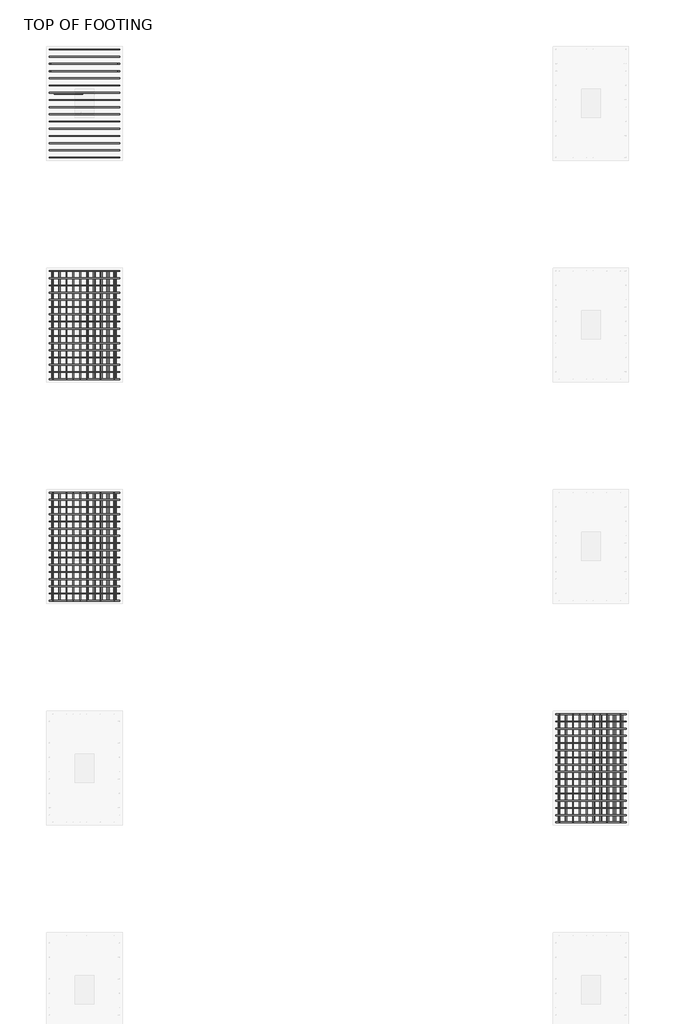
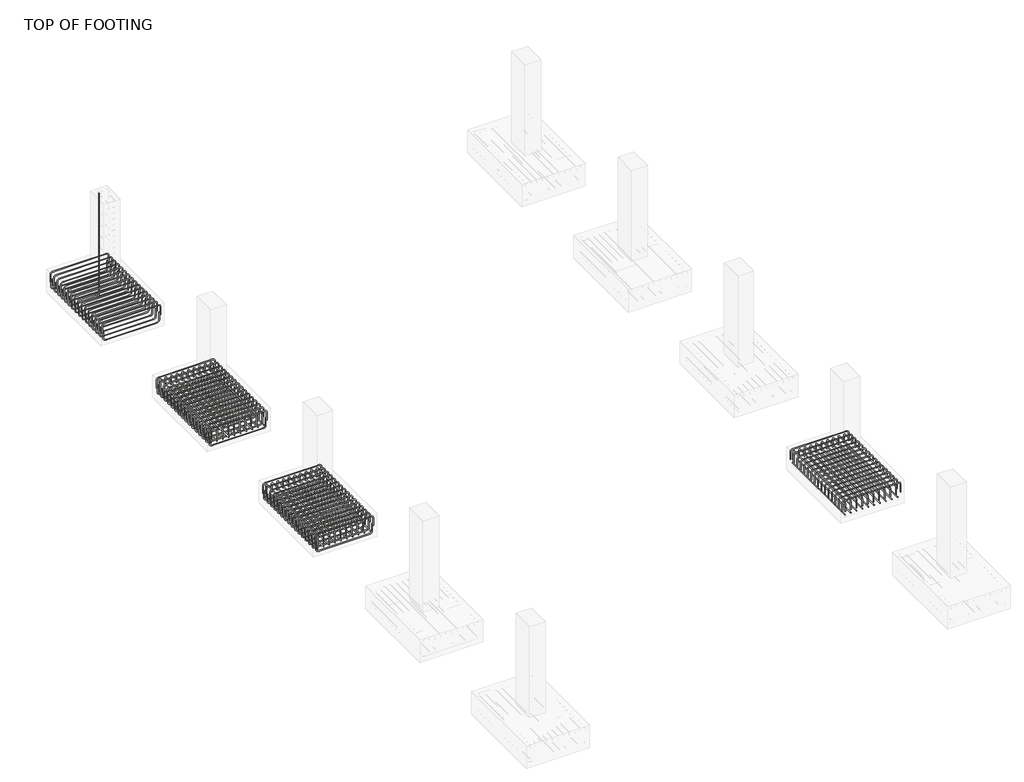
# One storey, part 3 of 8: 14 reinforcing bars.
"""IFC4 building model written with IfcOpenShell, lengths in millimetres."""

from ifc_helpers import new_model, si_unit, point, frame, origin, place, context, project, spatial, polyline, circle_curve, trimmed, segment, composite_curve, source, transform, mapped, element, save
from ifc_brep_helpers import swept_disk

model = new_model("IFC4")

# Units and contexts
model_context = context("Model", 3, world=origin())
ifc_project = project(units=[si_unit("LENGTHUNIT", "METRE", prefix="MILLI")], contexts=[model_context])

# Site, building, storey
site = spatial("IfcSite", under=ifc_project)
building = spatial("IfcBuilding", under=site)
storey = spatial("IfcBuildingStorey", under=building, Name="TOP OF FOOTING", Elevation=-1828.8)

# Reinforcing bars
placement = place(None, origin())
reinforcing_bar_shape = source(origin(), model_context, "Body", "SolidModel", [
    swept_disk(composite_curve([segment(polyline([(-11301.5220197, 16626.3508557, -2021.4413313), (-11301.5220197, 16626.3508557, -2168.7413313)]), True, "CONTINUOUS"), segment(trimmed(circle_curve(frame((-11347.8720197, 16626.3508557, -2168.7413313), z_axis=(0.0, 1.0, 0.0), x_axis=(46.350000000000364, 0.0, 0.0)), 46.35), [point((-11301.5220197, 16626.3508557, -2168.7413313))], [point((-11347.8720197, 16626.3508557, -2215.0913313))], True, "CARTESIAN"), True, "CONTINUOUS"), segment(polyline([(-11347.8720197, 16626.3508557, -2215.0913313), (-12320.167031, 16626.3508557, -2215.0913313)]), True, "CONTINUOUS"), segment(trimmed(circle_curve(frame((-12320.167031, 16626.3508557, -2168.7413313), z_axis=(0.0, 1.0, 0.0), x_axis=(0.0, 0.0, -46.34999999999991)), 46.35), [point((-12320.167031, 16626.3508557, -2215.0913313))], [point((-12366.517031, 16626.3508557, -2168.7413313))], True, "CARTESIAN"), True, "CONTINUOUS"), segment(polyline([(-12366.517031, 16626.3508557, -2168.7413313), (-12366.517031, 16626.3508557, -2021.4413313)]), True, "CONTINUOUS")], self_intersect=False), 6.35),
])
element("IfcReinforcingBar", 1, at=placement, inside=storey, context=model_context, shape_type="MappedRepresentation", body=[
    mapped(reinforcing_bar_shape, transform((0.0, 0.0, 0.0), x_axis=(1.0, 0.0, 0.0), y_axis=(0.0, 1.0, 0.0), z_axis=(0.0, 0.0, 1.0))),
    mapped(reinforcing_bar_shape, transform((0.0, -113.82, 0.0), x_axis=(1.0, 0.0, 0.0), y_axis=(0.0, 1.0, 0.0), z_axis=(0.0, 0.0, 1.0))),
    mapped(reinforcing_bar_shape, transform((0.0, -227.64, 0.0), x_axis=(1.0, 0.0, 0.0), y_axis=(0.0, 1.0, 0.0), z_axis=(0.0, 0.0, 1.0))),
    mapped(reinforcing_bar_shape, transform((0.0, -341.46, 0.0), x_axis=(1.0, 0.0, 0.0), y_axis=(0.0, 1.0, 0.0), z_axis=(0.0, 0.0, 1.0))),
    mapped(reinforcing_bar_shape, transform((0.0, -455.28, 0.0), x_axis=(1.0, 0.0, 0.0), y_axis=(0.0, 1.0, 0.0), z_axis=(0.0, 0.0, 1.0))),
    mapped(reinforcing_bar_shape, transform((0.0, -569.1, 0.0), x_axis=(1.0, 0.0, 0.0), y_axis=(0.0, 1.0, 0.0), z_axis=(0.0, 0.0, 1.0))),
    mapped(reinforcing_bar_shape, transform((0.0, -682.92, 0.0), x_axis=(1.0, 0.0, 0.0), y_axis=(0.0, 1.0, 0.0), z_axis=(0.0, 0.0, 1.0))),
    mapped(reinforcing_bar_shape, transform((0.0, -796.74, 0.0), x_axis=(1.0, 0.0, 0.0), y_axis=(0.0, 1.0, 0.0), z_axis=(0.0, 0.0, 1.0))),
    mapped(reinforcing_bar_shape, transform((0.0, -910.56, 0.0), x_axis=(1.0, 0.0, 0.0), y_axis=(0.0, 1.0, 0.0), z_axis=(0.0, 0.0, 1.0))),
    mapped(reinforcing_bar_shape, transform((0.0, -1024.38, 0.0), x_axis=(1.0, 0.0, 0.0), y_axis=(0.0, 1.0, 0.0), z_axis=(0.0, 0.0, 1.0))),
    mapped(reinforcing_bar_shape, transform((0.0, -1138.2, 0.0), x_axis=(1.0, 0.0, 0.0), y_axis=(0.0, 1.0, 0.0), z_axis=(0.0, 0.0, 1.0))),
    mapped(reinforcing_bar_shape, transform((0.0, -1252.02, 0.0), x_axis=(1.0, 0.0, 0.0), y_axis=(0.0, 1.0, 0.0), z_axis=(0.0, 0.0, 1.0))),
    mapped(reinforcing_bar_shape, transform((0.0, -1365.84, 0.0), x_axis=(1.0, 0.0, 0.0), y_axis=(0.0, 1.0, 0.0), z_axis=(0.0, 0.0, 1.0))),
    mapped(reinforcing_bar_shape, transform((0.0, -1479.66, 0.0), x_axis=(1.0, 0.0, 0.0), y_axis=(0.0, 1.0, 0.0), z_axis=(0.0, 0.0, 1.0))),
    mapped(reinforcing_bar_shape, transform((0.0, -1593.48, 0.0), x_axis=(1.0, 0.0, 0.0), y_axis=(0.0, 1.0, 0.0), z_axis=(0.0, 0.0, 1.0))),
    mapped(reinforcing_bar_shape, transform((0.0, -1707.3, 0.0), x_axis=(1.0, 0.0, 0.0), y_axis=(0.0, 1.0, 0.0), z_axis=(0.0, 0.0, 1.0))),
])
reinforcing_bar_2_shape = source(origin(), model_context, "Body", "SolidModel", [
    swept_disk(composite_curve([segment(polyline([(-12384.3374017, 16626.3508557, -2068.8), (-12384.3374017, 16626.3508557, -1921.5)]), True, "CONTINUOUS"), segment(trimmed(circle_curve(frame((-12337.9874017, 16626.3508557, -1921.5), z_axis=(0.0, 1.0, 0.0), x_axis=(-46.350000000000364, 0.0, 0.0)), 46.35), [point((-12384.3374017, 16626.3508557, -1921.5))], [point((-12337.9874017, 16626.3508557, -1875.15))], True, "CARTESIAN"), True, "CONTINUOUS"), segment(polyline([(-12337.9874017, 16626.3508557, -1875.15), (-11323.3874017, 16626.3508557, -1875.15)]), True, "CONTINUOUS"), segment(trimmed(circle_curve(frame((-11323.3874017, 16626.3508557, -1921.5), z_axis=(0.0, 1.0, 0.0), x_axis=(0.0, 0.0, 46.34999999999991)), 46.35), [point((-11323.3874017, 16626.3508557, -1875.15))], [point((-11277.0374017, 16626.3508557, -1921.5))], True, "CARTESIAN"), True, "CONTINUOUS"), segment(polyline([(-11277.0374017, 16626.3508557, -1921.5), (-11277.0374017, 16626.3508557, -2068.8)]), True, "CONTINUOUS")], self_intersect=False), 6.35),
])
element("IfcReinforcingBar", 2, at=placement, inside=storey, context=model_context, shape_type="MappedRepresentation", body=[
    mapped(reinforcing_bar_2_shape, transform((0.0, 0.0, 0.0), x_axis=(1.0, 0.0, 0.0), y_axis=(0.0, 1.0, 0.0), z_axis=(0.0, 0.0, 1.0))),
    mapped(reinforcing_bar_2_shape, transform((0.0, -113.82, 0.0), x_axis=(1.0, 0.0, 0.0), y_axis=(0.0, 1.0, 0.0), z_axis=(0.0, 0.0, 1.0))),
    mapped(reinforcing_bar_2_shape, transform((0.0, -227.64, 0.0), x_axis=(1.0, 0.0, 0.0), y_axis=(0.0, 1.0, 0.0), z_axis=(0.0, 0.0, 1.0))),
    mapped(reinforcing_bar_2_shape, transform((0.0, -341.46, 0.0), x_axis=(1.0, 0.0, 0.0), y_axis=(0.0, 1.0, 0.0), z_axis=(0.0, 0.0, 1.0))),
    mapped(reinforcing_bar_2_shape, transform((0.0, -455.28, 0.0), x_axis=(1.0, 0.0, 0.0), y_axis=(0.0, 1.0, 0.0), z_axis=(0.0, 0.0, 1.0))),
    mapped(reinforcing_bar_2_shape, transform((0.0, -569.1, 0.0), x_axis=(1.0, 0.0, 0.0), y_axis=(0.0, 1.0, 0.0), z_axis=(0.0, 0.0, 1.0))),
    mapped(reinforcing_bar_2_shape, transform((0.0, -682.92, 0.0), x_axis=(1.0, 0.0, 0.0), y_axis=(0.0, 1.0, 0.0), z_axis=(0.0, 0.0, 1.0))),
    mapped(reinforcing_bar_2_shape, transform((0.0, -796.74, 0.0), x_axis=(1.0, 0.0, 0.0), y_axis=(0.0, 1.0, 0.0), z_axis=(0.0, 0.0, 1.0))),
    mapped(reinforcing_bar_2_shape, transform((0.0, -910.56, 0.0), x_axis=(1.0, 0.0, 0.0), y_axis=(0.0, 1.0, 0.0), z_axis=(0.0, 0.0, 1.0))),
    mapped(reinforcing_bar_2_shape, transform((0.0, -1024.38, 0.0), x_axis=(1.0, 0.0, 0.0), y_axis=(0.0, 1.0, 0.0), z_axis=(0.0, 0.0, 1.0))),
    mapped(reinforcing_bar_2_shape, transform((0.0, -1138.2, 0.0), x_axis=(1.0, 0.0, 0.0), y_axis=(0.0, 1.0, 0.0), z_axis=(0.0, 0.0, 1.0))),
    mapped(reinforcing_bar_2_shape, transform((0.0, -1252.02, 0.0), x_axis=(1.0, 0.0, 0.0), y_axis=(0.0, 1.0, 0.0), z_axis=(0.0, 0.0, 1.0))),
    mapped(reinforcing_bar_2_shape, transform((0.0, -1365.84, 0.0), x_axis=(1.0, 0.0, 0.0), y_axis=(0.0, 1.0, 0.0), z_axis=(0.0, 0.0, 1.0))),
    mapped(reinforcing_bar_2_shape, transform((0.0, -1479.66, 0.0), x_axis=(1.0, 0.0, 0.0), y_axis=(0.0, 1.0, 0.0), z_axis=(0.0, 0.0, 1.0))),
    mapped(reinforcing_bar_2_shape, transform((0.0, -1593.48, 0.0), x_axis=(1.0, 0.0, 0.0), y_axis=(0.0, 1.0, 0.0), z_axis=(0.0, 0.0, 1.0))),
    mapped(reinforcing_bar_2_shape, transform((0.0, -1707.3, 0.0), x_axis=(1.0, 0.0, 0.0), y_axis=(0.0, 1.0, 0.0), z_axis=(0.0, 0.0, 1.0))),
])
element("IfcReinforcingBar", 3, at=placement, inside=storey, context=model_context, shape_type="SolidModel", body=[
    swept_disk(composite_curve([segment(polyline([(-11865.9367429, 15924.2508557, -40.0), (-11865.9367429, 15924.2508557, -2055.5685723)]), True, "CONTINUOUS"), segment(trimmed(circle_curve(frame((-11912.2867429, 15924.2508557, -2055.5685723), z_axis=(0.0, 1.0, 0.0), x_axis=(46.350000000000364, 0.0, 0.0)), 46.35), [point((-11865.9367429, 15924.2508557, -2055.5685723))], [point((-11912.2867429, 15924.2508557, -2101.9185723))], True, "CARTESIAN"), True, "CONTINUOUS"), segment(polyline([(-11912.2867429, 15924.2508557, -2101.9185723), (-12306.1579683, 15924.2508557, -2101.9185723)]), True, "CONTINUOUS")], self_intersect=False), 6.35),
])
reinforcing_bar_3_shape = source(origin(), model_context, "Body", "SolidModel", [
    swept_disk(composite_curve([segment(polyline([(-11301.5220197, 13126.3508557, -2021.4413313), (-11301.5220197, 13126.3508557, -2168.7413313)]), True, "CONTINUOUS"), segment(trimmed(circle_curve(frame((-11347.8720197, 13126.3508557, -2168.7413313), z_axis=(0.0, 1.0, 0.0), x_axis=(46.350000000000364, 0.0, 0.0)), 46.35), [point((-11301.5220197, 13126.3508557, -2168.7413313))], [point((-11347.8720197, 13126.3508557, -2215.0913313))], True, "CARTESIAN"), True, "CONTINUOUS"), segment(polyline([(-11347.8720197, 13126.3508557, -2215.0913313), (-12320.167031, 13126.3508557, -2215.0913313)]), True, "CONTINUOUS"), segment(trimmed(circle_curve(frame((-12320.167031, 13126.3508557, -2168.7413313), z_axis=(0.0, 1.0, 0.0), x_axis=(0.0, 0.0, -46.34999999999991)), 46.35), [point((-12320.167031, 13126.3508557, -2215.0913313))], [point((-12366.517031, 13126.3508557, -2168.7413313))], True, "CARTESIAN"), True, "CONTINUOUS"), segment(polyline([(-12366.517031, 13126.3508557, -2168.7413313), (-12366.517031, 13126.3508557, -2021.4413313)]), True, "CONTINUOUS")], self_intersect=False), 6.35),
])
element("IfcReinforcingBar", 4, at=placement, inside=storey, context=model_context, shape_type="MappedRepresentation", body=[
    mapped(reinforcing_bar_3_shape, transform((0.0, 0.0, 0.0), x_axis=(1.0, 0.0, 0.0), y_axis=(0.0, 1.0, 0.0), z_axis=(0.0, 0.0, 1.0))),
    mapped(reinforcing_bar_3_shape, transform((0.0, -113.82, 0.0), x_axis=(1.0, 0.0, 0.0), y_axis=(0.0, 1.0, 0.0), z_axis=(0.0, 0.0, 1.0))),
    mapped(reinforcing_bar_3_shape, transform((0.0, -227.64, 0.0), x_axis=(1.0, 0.0, 0.0), y_axis=(0.0, 1.0, 0.0), z_axis=(0.0, 0.0, 1.0))),
    mapped(reinforcing_bar_3_shape, transform((0.0, -341.46, 0.0), x_axis=(1.0, 0.0, 0.0), y_axis=(0.0, 1.0, 0.0), z_axis=(0.0, 0.0, 1.0))),
    mapped(reinforcing_bar_3_shape, transform((0.0, -455.28, 0.0), x_axis=(1.0, 0.0, 0.0), y_axis=(0.0, 1.0, 0.0), z_axis=(0.0, 0.0, 1.0))),
    mapped(reinforcing_bar_3_shape, transform((0.0, -569.1, 0.0), x_axis=(1.0, 0.0, 0.0), y_axis=(0.0, 1.0, 0.0), z_axis=(0.0, 0.0, 1.0))),
    mapped(reinforcing_bar_3_shape, transform((0.0, -682.92, 0.0), x_axis=(1.0, 0.0, 0.0), y_axis=(0.0, 1.0, 0.0), z_axis=(0.0, 0.0, 1.0))),
    mapped(reinforcing_bar_3_shape, transform((0.0, -796.74, 0.0), x_axis=(1.0, 0.0, 0.0), y_axis=(0.0, 1.0, 0.0), z_axis=(0.0, 0.0, 1.0))),
    mapped(reinforcing_bar_3_shape, transform((0.0, -910.56, 0.0), x_axis=(1.0, 0.0, 0.0), y_axis=(0.0, 1.0, 0.0), z_axis=(0.0, 0.0, 1.0))),
    mapped(reinforcing_bar_3_shape, transform((0.0, -1024.38, 0.0), x_axis=(1.0, 0.0, 0.0), y_axis=(0.0, 1.0, 0.0), z_axis=(0.0, 0.0, 1.0))),
    mapped(reinforcing_bar_3_shape, transform((0.0, -1138.2, 0.0), x_axis=(1.0, 0.0, 0.0), y_axis=(0.0, 1.0, 0.0), z_axis=(0.0, 0.0, 1.0))),
    mapped(reinforcing_bar_3_shape, transform((0.0, -1252.02, 0.0), x_axis=(1.0, 0.0, 0.0), y_axis=(0.0, 1.0, 0.0), z_axis=(0.0, 0.0, 1.0))),
    mapped(reinforcing_bar_3_shape, transform((0.0, -1365.84, 0.0), x_axis=(1.0, 0.0, 0.0), y_axis=(0.0, 1.0, 0.0), z_axis=(0.0, 0.0, 1.0))),
    mapped(reinforcing_bar_3_shape, transform((0.0, -1479.66, 0.0), x_axis=(1.0, 0.0, 0.0), y_axis=(0.0, 1.0, 0.0), z_axis=(0.0, 0.0, 1.0))),
    mapped(reinforcing_bar_3_shape, transform((0.0, -1593.48, 0.0), x_axis=(1.0, 0.0, 0.0), y_axis=(0.0, 1.0, 0.0), z_axis=(0.0, 0.0, 1.0))),
    mapped(reinforcing_bar_3_shape, transform((0.0, -1707.3, 0.0), x_axis=(1.0, 0.0, 0.0), y_axis=(0.0, 1.0, 0.0), z_axis=(0.0, 0.0, 1.0))),
])
reinforcing_bar_4_shape = source(origin(), model_context, "Body", "SolidModel", [
    swept_disk(composite_curve([segment(polyline([(-12384.3374017, 13126.3508557, -2068.8), (-12384.3374017, 13126.3508557, -1921.5)]), True, "CONTINUOUS"), segment(trimmed(circle_curve(frame((-12337.9874017, 13126.3508557, -1921.5), z_axis=(0.0, 1.0, 0.0), x_axis=(-46.350000000000364, 0.0, 0.0)), 46.35), [point((-12384.3374017, 13126.3508557, -1921.5))], [point((-12337.9874017, 13126.3508557, -1875.15))], True, "CARTESIAN"), True, "CONTINUOUS"), segment(polyline([(-12337.9874017, 13126.3508557, -1875.15), (-11323.3874017, 13126.3508557, -1875.15)]), True, "CONTINUOUS"), segment(trimmed(circle_curve(frame((-11323.3874017, 13126.3508557, -1921.5), z_axis=(0.0, 1.0, 0.0), x_axis=(0.0, 0.0, 46.34999999999991)), 46.35), [point((-11323.3874017, 13126.3508557, -1875.15))], [point((-11277.0374017, 13126.3508557, -1921.5))], True, "CARTESIAN"), True, "CONTINUOUS"), segment(polyline([(-11277.0374017, 13126.3508557, -1921.5), (-11277.0374017, 13126.3508557, -2068.8)]), True, "CONTINUOUS")], self_intersect=False), 6.35),
])
element("IfcReinforcingBar", 5, at=placement, inside=storey, context=model_context, shape_type="MappedRepresentation", body=[
    mapped(reinforcing_bar_4_shape, transform((0.0, 0.0, 0.0), x_axis=(1.0, 0.0, 0.0), y_axis=(0.0, 1.0, 0.0), z_axis=(0.0, 0.0, 1.0))),
    mapped(reinforcing_bar_4_shape, transform((0.0, -113.82, 0.0), x_axis=(1.0, 0.0, 0.0), y_axis=(0.0, 1.0, 0.0), z_axis=(0.0, 0.0, 1.0))),
    mapped(reinforcing_bar_4_shape, transform((0.0, -227.64, 0.0), x_axis=(1.0, 0.0, 0.0), y_axis=(0.0, 1.0, 0.0), z_axis=(0.0, 0.0, 1.0))),
    mapped(reinforcing_bar_4_shape, transform((0.0, -341.46, 0.0), x_axis=(1.0, 0.0, 0.0), y_axis=(0.0, 1.0, 0.0), z_axis=(0.0, 0.0, 1.0))),
    mapped(reinforcing_bar_4_shape, transform((0.0, -455.28, 0.0), x_axis=(1.0, 0.0, 0.0), y_axis=(0.0, 1.0, 0.0), z_axis=(0.0, 0.0, 1.0))),
    mapped(reinforcing_bar_4_shape, transform((0.0, -569.1, 0.0), x_axis=(1.0, 0.0, 0.0), y_axis=(0.0, 1.0, 0.0), z_axis=(0.0, 0.0, 1.0))),
    mapped(reinforcing_bar_4_shape, transform((0.0, -682.92, 0.0), x_axis=(1.0, 0.0, 0.0), y_axis=(0.0, 1.0, 0.0), z_axis=(0.0, 0.0, 1.0))),
    mapped(reinforcing_bar_4_shape, transform((0.0, -796.74, 0.0), x_axis=(1.0, 0.0, 0.0), y_axis=(0.0, 1.0, 0.0), z_axis=(0.0, 0.0, 1.0))),
    mapped(reinforcing_bar_4_shape, transform((0.0, -910.56, 0.0), x_axis=(1.0, 0.0, 0.0), y_axis=(0.0, 1.0, 0.0), z_axis=(0.0, 0.0, 1.0))),
    mapped(reinforcing_bar_4_shape, transform((0.0, -1024.38, 0.0), x_axis=(1.0, 0.0, 0.0), y_axis=(0.0, 1.0, 0.0), z_axis=(0.0, 0.0, 1.0))),
    mapped(reinforcing_bar_4_shape, transform((0.0, -1138.2, 0.0), x_axis=(1.0, 0.0, 0.0), y_axis=(0.0, 1.0, 0.0), z_axis=(0.0, 0.0, 1.0))),
    mapped(reinforcing_bar_4_shape, transform((0.0, -1252.02, 0.0), x_axis=(1.0, 0.0, 0.0), y_axis=(0.0, 1.0, 0.0), z_axis=(0.0, 0.0, 1.0))),
    mapped(reinforcing_bar_4_shape, transform((0.0, -1365.84, 0.0), x_axis=(1.0, 0.0, 0.0), y_axis=(0.0, 1.0, 0.0), z_axis=(0.0, 0.0, 1.0))),
    mapped(reinforcing_bar_4_shape, transform((0.0, -1479.66, 0.0), x_axis=(1.0, 0.0, 0.0), y_axis=(0.0, 1.0, 0.0), z_axis=(0.0, 0.0, 1.0))),
    mapped(reinforcing_bar_4_shape, transform((0.0, -1593.48, 0.0), x_axis=(1.0, 0.0, 0.0), y_axis=(0.0, 1.0, 0.0), z_axis=(0.0, 0.0, 1.0))),
    mapped(reinforcing_bar_4_shape, transform((0.0, -1707.3, 0.0), x_axis=(1.0, 0.0, 0.0), y_axis=(0.0, 1.0, 0.0), z_axis=(0.0, 0.0, 1.0))),
])
reinforcing_bar_5_shape = source(origin(), model_context, "Body", "SolidModel", [
    swept_disk(composite_curve([segment(polyline([(-12339.592709, 13132.7008557, -2155.1176129), (-12339.592709, 11412.7008557, -2155.1176129)]), True, "CONTINUOUS")], self_intersect=False), 6.35),
])
element("IfcReinforcingBar", 6, at=placement, inside=storey, context=model_context, shape_type="MappedRepresentation", body=[
    mapped(reinforcing_bar_5_shape, transform((0.0, 0.0, 0.0), x_axis=(1.0, 0.0, 0.0), y_axis=(0.0, 1.0, 0.0), z_axis=(0.0, 0.0, 1.0))),
    mapped(reinforcing_bar_5_shape, transform((111.602188, 0.0, 0.0), x_axis=(1.0, 0.0, 0.0), y_axis=(0.0, 1.0, 0.0), z_axis=(0.0, 0.0, 1.0))),
    mapped(reinforcing_bar_5_shape, transform((223.2043759, 0.0, 0.0), x_axis=(1.0, 0.0, 0.0), y_axis=(0.0, 1.0, 0.0), z_axis=(0.0, 0.0, 1.0))),
    mapped(reinforcing_bar_5_shape, transform((334.8065639, 0.0, 0.0), x_axis=(1.0, 0.0, 0.0), y_axis=(0.0, 1.0, 0.0), z_axis=(0.0, 0.0, 1.0))),
    mapped(reinforcing_bar_5_shape, transform((446.4087519, 0.0, 0.0), x_axis=(1.0, 0.0, 0.0), y_axis=(0.0, 1.0, 0.0), z_axis=(0.0, 0.0, 1.0))),
    mapped(reinforcing_bar_5_shape, transform((558.0109398, 0.0, 0.0), x_axis=(1.0, 0.0, 0.0), y_axis=(0.0, 1.0, 0.0), z_axis=(0.0, 0.0, 1.0))),
    mapped(reinforcing_bar_5_shape, transform((669.6131278, 0.0, 0.0), x_axis=(1.0, 0.0, 0.0), y_axis=(0.0, 1.0, 0.0), z_axis=(0.0, 0.0, 1.0))),
    mapped(reinforcing_bar_5_shape, transform((781.2153158, 0.0, 0.0), x_axis=(1.0, 0.0, 0.0), y_axis=(0.0, 1.0, 0.0), z_axis=(0.0, 0.0, 1.0))),
    mapped(reinforcing_bar_5_shape, transform((892.8175037, 0.0, 0.0), x_axis=(1.0, 0.0, 0.0), y_axis=(0.0, 1.0, 0.0), z_axis=(0.0, 0.0, 1.0))),
    mapped(reinforcing_bar_5_shape, transform((1004.4196917, 0.0, 0.0), x_axis=(1.0, 0.0, 0.0), y_axis=(0.0, 1.0, 0.0), z_axis=(0.0, 0.0, 1.0))),
])
reinforcing_bar_6_shape = source(origin(), model_context, "Body", "SolidModel", [
    swept_disk(composite_curve([segment(polyline([(-11364.2651981, 13126.3508557, -2094.6521303), (-11364.2651981, 13126.3508557, -1947.3521303)]), True, "CONTINUOUS"), segment(trimmed(circle_curve(frame((-11364.2651981, 13080.0008557, -1947.3521303), z_axis=(1.0, 0.0, 0.0), x_axis=(0.0, 46.350000000000364, 0.0)), 46.35), [point((-11364.2651981, 13126.3508557, -1947.3521303))], [point((-11364.2651981, 13080.0008557, -1901.0021303))], True, "CARTESIAN"), True, "CONTINUOUS"), segment(polyline([(-11364.2651981, 13080.0008557, -1901.0021303), (-11364.2651981, 11465.4008557, -1901.0021303)]), True, "CONTINUOUS"), segment(trimmed(circle_curve(frame((-11364.2651981, 11465.4008557, -1947.3521303), z_axis=(1.0, 0.0, 0.0), x_axis=(0.0, 0.0, 46.34999999999991)), 46.35), [point((-11364.2651981, 11465.4008557, -1901.0021303))], [point((-11364.2651981, 11419.0508557, -1947.3521303))], True, "CARTESIAN"), True, "CONTINUOUS"), segment(polyline([(-11364.2651981, 11419.0508557, -1947.3521303), (-11364.2651981, 11419.0508557, -2094.6521303)]), True, "CONTINUOUS")], self_intersect=False), 6.35),
])
element("IfcReinforcingBar", 7, at=placement, inside=storey, context=model_context, shape_type="MappedRepresentation", body=[
    mapped(reinforcing_bar_6_shape, transform((0.0, 0.0, 0.0), x_axis=(1.0, 0.0, 0.0), y_axis=(0.0, 1.0, 0.0), z_axis=(0.0, 0.0, 1.0))),
    mapped(reinforcing_bar_6_shape, transform((-107.1680233, 0.0, 0.0), x_axis=(1.0, 0.0, 0.0), y_axis=(0.0, 1.0, 0.0), z_axis=(0.0, 0.0, 1.0))),
    mapped(reinforcing_bar_6_shape, transform((-214.3360466, 0.0, 0.0), x_axis=(1.0, 0.0, 0.0), y_axis=(0.0, 1.0, 0.0), z_axis=(0.0, 0.0, 1.0))),
    mapped(reinforcing_bar_6_shape, transform((-321.5040699, 0.0, 0.0), x_axis=(1.0, 0.0, 0.0), y_axis=(0.0, 1.0, 0.0), z_axis=(0.0, 0.0, 1.0))),
    mapped(reinforcing_bar_6_shape, transform((-428.6720932, 0.0, 0.0), x_axis=(1.0, 0.0, 0.0), y_axis=(0.0, 1.0, 0.0), z_axis=(0.0, 0.0, 1.0))),
    mapped(reinforcing_bar_6_shape, transform((-535.8401165, 0.0, 0.0), x_axis=(1.0, 0.0, 0.0), y_axis=(0.0, 1.0, 0.0), z_axis=(0.0, 0.0, 1.0))),
    mapped(reinforcing_bar_6_shape, transform((-643.0081398, 0.0, 0.0), x_axis=(1.0, 0.0, 0.0), y_axis=(0.0, 1.0, 0.0), z_axis=(0.0, 0.0, 1.0))),
    mapped(reinforcing_bar_6_shape, transform((-750.176163, 0.0, 0.0), x_axis=(1.0, 0.0, 0.0), y_axis=(0.0, 1.0, 0.0), z_axis=(0.0, 0.0, 1.0))),
    mapped(reinforcing_bar_6_shape, transform((-857.3441863, 0.0, 0.0), x_axis=(1.0, 0.0, 0.0), y_axis=(0.0, 1.0, 0.0), z_axis=(0.0, 0.0, 1.0))),
    mapped(reinforcing_bar_6_shape, transform((-964.5122096, 0.0, 0.0), x_axis=(1.0, 0.0, 0.0), y_axis=(0.0, 1.0, 0.0), z_axis=(0.0, 0.0, 1.0))),
])
reinforcing_bar_7_shape = source(origin(), model_context, "Body", "SolidModel", [
    swept_disk(composite_curve([segment(polyline([(-11301.5220197, 9626.3508557, -2021.4413313), (-11301.5220197, 9626.3508557, -2168.7413313)]), True, "CONTINUOUS"), segment(trimmed(circle_curve(frame((-11347.8720197, 9626.3508557, -2168.7413313), z_axis=(0.0, 1.0, 0.0), x_axis=(46.350000000000364, 0.0, 0.0)), 46.35), [point((-11301.5220197, 9626.3508557, -2168.7413313))], [point((-11347.8720197, 9626.3508557, -2215.0913313))], True, "CARTESIAN"), True, "CONTINUOUS"), segment(polyline([(-11347.8720197, 9626.3508557, -2215.0913313), (-12320.167031, 9626.3508557, -2215.0913313)]), True, "CONTINUOUS"), segment(trimmed(circle_curve(frame((-12320.167031, 9626.3508557, -2168.7413313), z_axis=(0.0, 1.0, 0.0), x_axis=(0.0, 0.0, -46.34999999999991)), 46.35), [point((-12320.167031, 9626.3508557, -2215.0913313))], [point((-12366.517031, 9626.3508557, -2168.7413313))], True, "CARTESIAN"), True, "CONTINUOUS"), segment(polyline([(-12366.517031, 9626.3508557, -2168.7413313), (-12366.517031, 9626.3508557, -2021.4413313)]), True, "CONTINUOUS")], self_intersect=False), 6.35),
])
element("IfcReinforcingBar", 8, at=placement, inside=storey, context=model_context, shape_type="MappedRepresentation", body=[
    mapped(reinforcing_bar_7_shape, transform((0.0, 0.0, 0.0), x_axis=(1.0, 0.0, 0.0), y_axis=(0.0, 1.0, 0.0), z_axis=(0.0, 0.0, 1.0))),
    mapped(reinforcing_bar_7_shape, transform((0.0, -113.82, 0.0), x_axis=(1.0, 0.0, 0.0), y_axis=(0.0, 1.0, 0.0), z_axis=(0.0, 0.0, 1.0))),
    mapped(reinforcing_bar_7_shape, transform((0.0, -227.64, 0.0), x_axis=(1.0, 0.0, 0.0), y_axis=(0.0, 1.0, 0.0), z_axis=(0.0, 0.0, 1.0))),
    mapped(reinforcing_bar_7_shape, transform((0.0, -341.46, 0.0), x_axis=(1.0, 0.0, 0.0), y_axis=(0.0, 1.0, 0.0), z_axis=(0.0, 0.0, 1.0))),
    mapped(reinforcing_bar_7_shape, transform((0.0, -455.28, 0.0), x_axis=(1.0, 0.0, 0.0), y_axis=(0.0, 1.0, 0.0), z_axis=(0.0, 0.0, 1.0))),
    mapped(reinforcing_bar_7_shape, transform((0.0, -569.1, 0.0), x_axis=(1.0, 0.0, 0.0), y_axis=(0.0, 1.0, 0.0), z_axis=(0.0, 0.0, 1.0))),
    mapped(reinforcing_bar_7_shape, transform((0.0, -682.92, 0.0), x_axis=(1.0, 0.0, 0.0), y_axis=(0.0, 1.0, 0.0), z_axis=(0.0, 0.0, 1.0))),
    mapped(reinforcing_bar_7_shape, transform((0.0, -796.74, 0.0), x_axis=(1.0, 0.0, 0.0), y_axis=(0.0, 1.0, 0.0), z_axis=(0.0, 0.0, 1.0))),
    mapped(reinforcing_bar_7_shape, transform((0.0, -910.56, 0.0), x_axis=(1.0, 0.0, 0.0), y_axis=(0.0, 1.0, 0.0), z_axis=(0.0, 0.0, 1.0))),
    mapped(reinforcing_bar_7_shape, transform((0.0, -1024.38, 0.0), x_axis=(1.0, 0.0, 0.0), y_axis=(0.0, 1.0, 0.0), z_axis=(0.0, 0.0, 1.0))),
    mapped(reinforcing_bar_7_shape, transform((0.0, -1138.2, 0.0), x_axis=(1.0, 0.0, 0.0), y_axis=(0.0, 1.0, 0.0), z_axis=(0.0, 0.0, 1.0))),
    mapped(reinforcing_bar_7_shape, transform((0.0, -1252.02, 0.0), x_axis=(1.0, 0.0, 0.0), y_axis=(0.0, 1.0, 0.0), z_axis=(0.0, 0.0, 1.0))),
    mapped(reinforcing_bar_7_shape, transform((0.0, -1365.84, 0.0), x_axis=(1.0, 0.0, 0.0), y_axis=(0.0, 1.0, 0.0), z_axis=(0.0, 0.0, 1.0))),
    mapped(reinforcing_bar_7_shape, transform((0.0, -1479.66, 0.0), x_axis=(1.0, 0.0, 0.0), y_axis=(0.0, 1.0, 0.0), z_axis=(0.0, 0.0, 1.0))),
    mapped(reinforcing_bar_7_shape, transform((0.0, -1593.48, 0.0), x_axis=(1.0, 0.0, 0.0), y_axis=(0.0, 1.0, 0.0), z_axis=(0.0, 0.0, 1.0))),
    mapped(reinforcing_bar_7_shape, transform((0.0, -1707.3, 0.0), x_axis=(1.0, 0.0, 0.0), y_axis=(0.0, 1.0, 0.0), z_axis=(0.0, 0.0, 1.0))),
])
reinforcing_bar_8_shape = source(origin(), model_context, "Body", "SolidModel", [
    swept_disk(composite_curve([segment(polyline([(-12384.3374017, 9626.3508557, -2068.8), (-12384.3374017, 9626.3508557, -1921.5)]), True, "CONTINUOUS"), segment(trimmed(circle_curve(frame((-12337.9874017, 9626.3508557, -1921.5), z_axis=(0.0, 1.0, 0.0), x_axis=(-46.350000000000364, 0.0, 0.0)), 46.35), [point((-12384.3374017, 9626.3508557, -1921.5))], [point((-12337.9874017, 9626.3508557, -1875.15))], True, "CARTESIAN"), True, "CONTINUOUS"), segment(polyline([(-12337.9874017, 9626.3508557, -1875.15), (-11323.3874017, 9626.3508557, -1875.15)]), True, "CONTINUOUS"), segment(trimmed(circle_curve(frame((-11323.3874017, 9626.3508557, -1921.5), z_axis=(0.0, 1.0, 0.0), x_axis=(0.0, 0.0, 46.34999999999991)), 46.35), [point((-11323.3874017, 9626.3508557, -1875.15))], [point((-11277.0374017, 9626.3508557, -1921.5))], True, "CARTESIAN"), True, "CONTINUOUS"), segment(polyline([(-11277.0374017, 9626.3508557, -1921.5), (-11277.0374017, 9626.3508557, -2068.8)]), True, "CONTINUOUS")], self_intersect=False), 6.35),
])
element("IfcReinforcingBar", 9, at=placement, inside=storey, context=model_context, shape_type="MappedRepresentation", body=[
    mapped(reinforcing_bar_8_shape, transform((0.0, 0.0, 0.0), x_axis=(1.0, 0.0, 0.0), y_axis=(0.0, 1.0, 0.0), z_axis=(0.0, 0.0, 1.0))),
    mapped(reinforcing_bar_8_shape, transform((0.0, -113.82, 0.0), x_axis=(1.0, 0.0, 0.0), y_axis=(0.0, 1.0, 0.0), z_axis=(0.0, 0.0, 1.0))),
    mapped(reinforcing_bar_8_shape, transform((0.0, -227.64, 0.0), x_axis=(1.0, 0.0, 0.0), y_axis=(0.0, 1.0, 0.0), z_axis=(0.0, 0.0, 1.0))),
    mapped(reinforcing_bar_8_shape, transform((0.0, -341.46, 0.0), x_axis=(1.0, 0.0, 0.0), y_axis=(0.0, 1.0, 0.0), z_axis=(0.0, 0.0, 1.0))),
    mapped(reinforcing_bar_8_shape, transform((0.0, -455.28, 0.0), x_axis=(1.0, 0.0, 0.0), y_axis=(0.0, 1.0, 0.0), z_axis=(0.0, 0.0, 1.0))),
    mapped(reinforcing_bar_8_shape, transform((0.0, -569.1, 0.0), x_axis=(1.0, 0.0, 0.0), y_axis=(0.0, 1.0, 0.0), z_axis=(0.0, 0.0, 1.0))),
    mapped(reinforcing_bar_8_shape, transform((0.0, -682.92, 0.0), x_axis=(1.0, 0.0, 0.0), y_axis=(0.0, 1.0, 0.0), z_axis=(0.0, 0.0, 1.0))),
    mapped(reinforcing_bar_8_shape, transform((0.0, -796.74, 0.0), x_axis=(1.0, 0.0, 0.0), y_axis=(0.0, 1.0, 0.0), z_axis=(0.0, 0.0, 1.0))),
    mapped(reinforcing_bar_8_shape, transform((0.0, -910.56, 0.0), x_axis=(1.0, 0.0, 0.0), y_axis=(0.0, 1.0, 0.0), z_axis=(0.0, 0.0, 1.0))),
    mapped(reinforcing_bar_8_shape, transform((0.0, -1024.38, 0.0), x_axis=(1.0, 0.0, 0.0), y_axis=(0.0, 1.0, 0.0), z_axis=(0.0, 0.0, 1.0))),
    mapped(reinforcing_bar_8_shape, transform((0.0, -1138.2, 0.0), x_axis=(1.0, 0.0, 0.0), y_axis=(0.0, 1.0, 0.0), z_axis=(0.0, 0.0, 1.0))),
    mapped(reinforcing_bar_8_shape, transform((0.0, -1252.02, 0.0), x_axis=(1.0, 0.0, 0.0), y_axis=(0.0, 1.0, 0.0), z_axis=(0.0, 0.0, 1.0))),
    mapped(reinforcing_bar_8_shape, transform((0.0, -1365.84, 0.0), x_axis=(1.0, 0.0, 0.0), y_axis=(0.0, 1.0, 0.0), z_axis=(0.0, 0.0, 1.0))),
    mapped(reinforcing_bar_8_shape, transform((0.0, -1479.66, 0.0), x_axis=(1.0, 0.0, 0.0), y_axis=(0.0, 1.0, 0.0), z_axis=(0.0, 0.0, 1.0))),
    mapped(reinforcing_bar_8_shape, transform((0.0, -1593.48, 0.0), x_axis=(1.0, 0.0, 0.0), y_axis=(0.0, 1.0, 0.0), z_axis=(0.0, 0.0, 1.0))),
    mapped(reinforcing_bar_8_shape, transform((0.0, -1707.3, 0.0), x_axis=(1.0, 0.0, 0.0), y_axis=(0.0, 1.0, 0.0), z_axis=(0.0, 0.0, 1.0))),
])
reinforcing_bar_9_shape = source(origin(), model_context, "Body", "SolidModel", [
    swept_disk(composite_curve([segment(polyline([(-12339.592709, 9632.7008557, -2155.1176129), (-12339.592709, 7912.7008557, -2155.1176129)]), True, "CONTINUOUS")], self_intersect=False), 6.35),
])
element("IfcReinforcingBar", 10, at=placement, inside=storey, context=model_context, shape_type="MappedRepresentation", body=[
    mapped(reinforcing_bar_9_shape, transform((0.0, 0.0, 0.0), x_axis=(1.0, 0.0, 0.0), y_axis=(0.0, 1.0, 0.0), z_axis=(0.0, 0.0, 1.0))),
    mapped(reinforcing_bar_9_shape, transform((111.602188, 0.0, 0.0), x_axis=(1.0, 0.0, 0.0), y_axis=(0.0, 1.0, 0.0), z_axis=(0.0, 0.0, 1.0))),
    mapped(reinforcing_bar_9_shape, transform((223.2043759, 0.0, 0.0), x_axis=(1.0, 0.0, 0.0), y_axis=(0.0, 1.0, 0.0), z_axis=(0.0, 0.0, 1.0))),
    mapped(reinforcing_bar_9_shape, transform((334.8065639, 0.0, 0.0), x_axis=(1.0, 0.0, 0.0), y_axis=(0.0, 1.0, 0.0), z_axis=(0.0, 0.0, 1.0))),
    mapped(reinforcing_bar_9_shape, transform((446.4087519, 0.0, 0.0), x_axis=(1.0, 0.0, 0.0), y_axis=(0.0, 1.0, 0.0), z_axis=(0.0, 0.0, 1.0))),
    mapped(reinforcing_bar_9_shape, transform((558.0109398, 0.0, 0.0), x_axis=(1.0, 0.0, 0.0), y_axis=(0.0, 1.0, 0.0), z_axis=(0.0, 0.0, 1.0))),
    mapped(reinforcing_bar_9_shape, transform((669.6131278, 0.0, 0.0), x_axis=(1.0, 0.0, 0.0), y_axis=(0.0, 1.0, 0.0), z_axis=(0.0, 0.0, 1.0))),
    mapped(reinforcing_bar_9_shape, transform((781.2153158, 0.0, 0.0), x_axis=(1.0, 0.0, 0.0), y_axis=(0.0, 1.0, 0.0), z_axis=(0.0, 0.0, 1.0))),
    mapped(reinforcing_bar_9_shape, transform((892.8175037, 0.0, 0.0), x_axis=(1.0, 0.0, 0.0), y_axis=(0.0, 1.0, 0.0), z_axis=(0.0, 0.0, 1.0))),
    mapped(reinforcing_bar_9_shape, transform((1004.4196917, 0.0, 0.0), x_axis=(1.0, 0.0, 0.0), y_axis=(0.0, 1.0, 0.0), z_axis=(0.0, 0.0, 1.0))),
])
reinforcing_bar_10_shape = source(origin(), model_context, "Body", "SolidModel", [
    swept_disk(composite_curve([segment(polyline([(-11364.2651981, 9626.3508557, -2094.6521303), (-11364.2651981, 9626.3508557, -1947.3521303)]), True, "CONTINUOUS"), segment(trimmed(circle_curve(frame((-11364.2651981, 9580.0008557, -1947.3521303), z_axis=(1.0, 0.0, 0.0), x_axis=(0.0, 46.350000000000364, 0.0)), 46.35), [point((-11364.2651981, 9626.3508557, -1947.3521303))], [point((-11364.2651981, 9580.0008557, -1901.0021303))], True, "CARTESIAN"), True, "CONTINUOUS"), segment(polyline([(-11364.2651981, 9580.0008557, -1901.0021303), (-11364.2651981, 7965.4008557, -1901.0021303)]), True, "CONTINUOUS"), segment(trimmed(circle_curve(frame((-11364.2651981, 7965.4008557, -1947.3521303), z_axis=(1.0, 0.0, 0.0), x_axis=(0.0, 0.0, 46.34999999999991)), 46.35), [point((-11364.2651981, 7965.4008557, -1901.0021303))], [point((-11364.2651981, 7919.0508557, -1947.3521303))], True, "CARTESIAN"), True, "CONTINUOUS"), segment(polyline([(-11364.2651981, 7919.0508557, -1947.3521303), (-11364.2651981, 7919.0508557, -2094.6521303)]), True, "CONTINUOUS")], self_intersect=False), 6.35),
])
element("IfcReinforcingBar", 11, at=placement, inside=storey, context=model_context, shape_type="MappedRepresentation", body=[
    mapped(reinforcing_bar_10_shape, transform((0.0, 0.0, 0.0), x_axis=(1.0, 0.0, 0.0), y_axis=(0.0, 1.0, 0.0), z_axis=(0.0, 0.0, 1.0))),
    mapped(reinforcing_bar_10_shape, transform((-107.1680233, 0.0, 0.0), x_axis=(1.0, 0.0, 0.0), y_axis=(0.0, 1.0, 0.0), z_axis=(0.0, 0.0, 1.0))),
    mapped(reinforcing_bar_10_shape, transform((-214.3360466, 0.0, 0.0), x_axis=(1.0, 0.0, 0.0), y_axis=(0.0, 1.0, 0.0), z_axis=(0.0, 0.0, 1.0))),
    mapped(reinforcing_bar_10_shape, transform((-321.5040699, 0.0, 0.0), x_axis=(1.0, 0.0, 0.0), y_axis=(0.0, 1.0, 0.0), z_axis=(0.0, 0.0, 1.0))),
    mapped(reinforcing_bar_10_shape, transform((-428.6720932, 0.0, 0.0), x_axis=(1.0, 0.0, 0.0), y_axis=(0.0, 1.0, 0.0), z_axis=(0.0, 0.0, 1.0))),
    mapped(reinforcing_bar_10_shape, transform((-535.8401165, 0.0, 0.0), x_axis=(1.0, 0.0, 0.0), y_axis=(0.0, 1.0, 0.0), z_axis=(0.0, 0.0, 1.0))),
    mapped(reinforcing_bar_10_shape, transform((-643.0081398, 0.0, 0.0), x_axis=(1.0, 0.0, 0.0), y_axis=(0.0, 1.0, 0.0), z_axis=(0.0, 0.0, 1.0))),
    mapped(reinforcing_bar_10_shape, transform((-750.176163, 0.0, 0.0), x_axis=(1.0, 0.0, 0.0), y_axis=(0.0, 1.0, 0.0), z_axis=(0.0, 0.0, 1.0))),
    mapped(reinforcing_bar_10_shape, transform((-857.3441863, 0.0, 0.0), x_axis=(1.0, 0.0, 0.0), y_axis=(0.0, 1.0, 0.0), z_axis=(0.0, 0.0, 1.0))),
    mapped(reinforcing_bar_10_shape, transform((-964.5122096, 0.0, 0.0), x_axis=(1.0, 0.0, 0.0), y_axis=(0.0, 1.0, 0.0), z_axis=(0.0, 0.0, 1.0))),
])
reinforcing_bar_11_shape = source(origin(), model_context, "Body", "SolidModel", [
    swept_disk(composite_curve([segment(polyline([(-4384.3374017, 6126.3508557, -2068.8), (-4384.3374017, 6126.3508557, -1921.5)]), True, "CONTINUOUS"), segment(trimmed(circle_curve(frame((-4337.9874017, 6126.3508557, -1921.5), z_axis=(0.0, 1.0, 0.0), x_axis=(-46.349999999999454, 0.0, 0.0)), 46.35), [point((-4384.3374017, 6126.3508557, -1921.5))], [point((-4337.9874017, 6126.3508557, -1875.15))], True, "CARTESIAN"), True, "CONTINUOUS"), segment(polyline([(-4337.9874017, 6126.3508557, -1875.15), (-3323.3874017, 6126.3508557, -1875.15)]), True, "CONTINUOUS"), segment(trimmed(circle_curve(frame((-3323.3874017, 6126.3508557, -1921.5), z_axis=(0.0, 1.0, 0.0), x_axis=(0.0, 0.0, 46.34999999999991)), 46.35), [point((-3323.3874017, 6126.3508557, -1875.15))], [point((-3277.0374017, 6126.3508557, -1921.5))], True, "CARTESIAN"), True, "CONTINUOUS"), segment(polyline([(-3277.0374017, 6126.3508557, -1921.5), (-3277.0374017, 6126.3508557, -2068.8)]), True, "CONTINUOUS")], self_intersect=False), 6.35),
])
element("IfcReinforcingBar", 12, at=placement, inside=storey, context=model_context, shape_type="MappedRepresentation", body=[
    mapped(reinforcing_bar_11_shape, transform((0.0, 0.0, 0.0), x_axis=(1.0, 0.0, 0.0), y_axis=(0.0, 1.0, 0.0), z_axis=(0.0, 0.0, 1.0))),
    mapped(reinforcing_bar_11_shape, transform((0.0, -113.82, 0.0), x_axis=(1.0, 0.0, 0.0), y_axis=(0.0, 1.0, 0.0), z_axis=(0.0, 0.0, 1.0))),
    mapped(reinforcing_bar_11_shape, transform((0.0, -227.64, 0.0), x_axis=(1.0, 0.0, 0.0), y_axis=(0.0, 1.0, 0.0), z_axis=(0.0, 0.0, 1.0))),
    mapped(reinforcing_bar_11_shape, transform((0.0, -341.46, 0.0), x_axis=(1.0, 0.0, 0.0), y_axis=(0.0, 1.0, 0.0), z_axis=(0.0, 0.0, 1.0))),
    mapped(reinforcing_bar_11_shape, transform((0.0, -455.28, 0.0), x_axis=(1.0, 0.0, 0.0), y_axis=(0.0, 1.0, 0.0), z_axis=(0.0, 0.0, 1.0))),
    mapped(reinforcing_bar_11_shape, transform((0.0, -569.1, 0.0), x_axis=(1.0, 0.0, 0.0), y_axis=(0.0, 1.0, 0.0), z_axis=(0.0, 0.0, 1.0))),
    mapped(reinforcing_bar_11_shape, transform((0.0, -682.92, 0.0), x_axis=(1.0, 0.0, 0.0), y_axis=(0.0, 1.0, 0.0), z_axis=(0.0, 0.0, 1.0))),
    mapped(reinforcing_bar_11_shape, transform((0.0, -796.74, 0.0), x_axis=(1.0, 0.0, 0.0), y_axis=(0.0, 1.0, 0.0), z_axis=(0.0, 0.0, 1.0))),
    mapped(reinforcing_bar_11_shape, transform((0.0, -910.56, 0.0), x_axis=(1.0, 0.0, 0.0), y_axis=(0.0, 1.0, 0.0), z_axis=(0.0, 0.0, 1.0))),
    mapped(reinforcing_bar_11_shape, transform((0.0, -1024.38, 0.0), x_axis=(1.0, 0.0, 0.0), y_axis=(0.0, 1.0, 0.0), z_axis=(0.0, 0.0, 1.0))),
    mapped(reinforcing_bar_11_shape, transform((0.0, -1138.2, 0.0), x_axis=(1.0, 0.0, 0.0), y_axis=(0.0, 1.0, 0.0), z_axis=(0.0, 0.0, 1.0))),
    mapped(reinforcing_bar_11_shape, transform((0.0, -1252.02, 0.0), x_axis=(1.0, 0.0, 0.0), y_axis=(0.0, 1.0, 0.0), z_axis=(0.0, 0.0, 1.0))),
    mapped(reinforcing_bar_11_shape, transform((0.0, -1365.84, 0.0), x_axis=(1.0, 0.0, 0.0), y_axis=(0.0, 1.0, 0.0), z_axis=(0.0, 0.0, 1.0))),
    mapped(reinforcing_bar_11_shape, transform((0.0, -1479.66, 0.0), x_axis=(1.0, 0.0, 0.0), y_axis=(0.0, 1.0, 0.0), z_axis=(0.0, 0.0, 1.0))),
    mapped(reinforcing_bar_11_shape, transform((0.0, -1593.48, 0.0), x_axis=(1.0, 0.0, 0.0), y_axis=(0.0, 1.0, 0.0), z_axis=(0.0, 0.0, 1.0))),
    mapped(reinforcing_bar_11_shape, transform((0.0, -1707.3, 0.0), x_axis=(1.0, 0.0, 0.0), y_axis=(0.0, 1.0, 0.0), z_axis=(0.0, 0.0, 1.0))),
])
reinforcing_bar_12_shape = source(origin(), model_context, "Body", "SolidModel", [
    swept_disk(composite_curve([segment(polyline([(-4339.592709, 6132.7008557, -2155.1176129), (-4339.592709, 4412.7008557, -2155.1176129)]), True, "CONTINUOUS")], self_intersect=False), 6.35),
])
element("IfcReinforcingBar", 13, at=placement, inside=storey, context=model_context, shape_type="MappedRepresentation", body=[
    mapped(reinforcing_bar_12_shape, transform((0.0, 0.0, 0.0), x_axis=(1.0, 0.0, 0.0), y_axis=(0.0, 1.0, 0.0), z_axis=(0.0, 0.0, 1.0))),
    mapped(reinforcing_bar_12_shape, transform((111.602188, 0.0, 0.0), x_axis=(1.0, 0.0, 0.0), y_axis=(0.0, 1.0, 0.0), z_axis=(0.0, 0.0, 1.0))),
    mapped(reinforcing_bar_12_shape, transform((223.2043759, 0.0, 0.0), x_axis=(1.0, 0.0, 0.0), y_axis=(0.0, 1.0, 0.0), z_axis=(0.0, 0.0, 1.0))),
    mapped(reinforcing_bar_12_shape, transform((334.8065639, 0.0, 0.0), x_axis=(1.0, 0.0, 0.0), y_axis=(0.0, 1.0, 0.0), z_axis=(0.0, 0.0, 1.0))),
    mapped(reinforcing_bar_12_shape, transform((446.4087519, 0.0, 0.0), x_axis=(1.0, 0.0, 0.0), y_axis=(0.0, 1.0, 0.0), z_axis=(0.0, 0.0, 1.0))),
    mapped(reinforcing_bar_12_shape, transform((558.0109398, 0.0, 0.0), x_axis=(1.0, 0.0, 0.0), y_axis=(0.0, 1.0, 0.0), z_axis=(0.0, 0.0, 1.0))),
    mapped(reinforcing_bar_12_shape, transform((669.6131278, 0.0, 0.0), x_axis=(1.0, 0.0, 0.0), y_axis=(0.0, 1.0, 0.0), z_axis=(0.0, 0.0, 1.0))),
    mapped(reinforcing_bar_12_shape, transform((781.2153158, 0.0, 0.0), x_axis=(1.0, 0.0, 0.0), y_axis=(0.0, 1.0, 0.0), z_axis=(0.0, 0.0, 1.0))),
    mapped(reinforcing_bar_12_shape, transform((892.8175037, 0.0, 0.0), x_axis=(1.0, 0.0, 0.0), y_axis=(0.0, 1.0, 0.0), z_axis=(0.0, 0.0, 1.0))),
    mapped(reinforcing_bar_12_shape, transform((1004.4196917, 0.0, 0.0), x_axis=(1.0, 0.0, 0.0), y_axis=(0.0, 1.0, 0.0), z_axis=(0.0, 0.0, 1.0))),
])
reinforcing_bar_13_shape = source(origin(), model_context, "Body", "SolidModel", [
    swept_disk(composite_curve([segment(polyline([(-3364.2651981, 6126.3508557, -2094.6521303), (-3364.2651981, 6126.3508557, -1947.3521303)]), True, "CONTINUOUS"), segment(trimmed(circle_curve(frame((-3364.2651981, 6080.0008557, -1947.3521303), z_axis=(1.0, 0.0, 0.0), x_axis=(0.0, 46.349999999999454, 0.0)), 46.35), [point((-3364.2651981, 6126.3508557, -1947.3521303))], [point((-3364.2651981, 6080.0008557, -1901.0021303))], True, "CARTESIAN"), True, "CONTINUOUS"), segment(polyline([(-3364.2651981, 6080.0008557, -1901.0021303), (-3364.2651981, 4465.4008557, -1901.0021303)]), True, "CONTINUOUS"), segment(trimmed(circle_curve(frame((-3364.2651981, 4465.4008557, -1947.3521303), z_axis=(1.0, 0.0, 0.0), x_axis=(0.0, 0.0, 46.34999999999991)), 46.35), [point((-3364.2651981, 4465.4008557, -1901.0021303))], [point((-3364.2651981, 4419.0508557, -1947.3521303))], True, "CARTESIAN"), True, "CONTINUOUS"), segment(polyline([(-3364.2651981, 4419.0508557, -1947.3521303), (-3364.2651981, 4419.0508557, -2094.6521303)]), True, "CONTINUOUS")], self_intersect=False), 6.35),
])
element("IfcReinforcingBar", 14, at=placement, inside=storey, context=model_context, shape_type="MappedRepresentation", body=[
    mapped(reinforcing_bar_13_shape, transform((0.0, 0.0, 0.0), x_axis=(1.0, 0.0, 0.0), y_axis=(0.0, 1.0, 0.0), z_axis=(0.0, 0.0, 1.0))),
    mapped(reinforcing_bar_13_shape, transform((-107.1680233, 0.0, 0.0), x_axis=(1.0, 0.0, 0.0), y_axis=(0.0, 1.0, 0.0), z_axis=(0.0, 0.0, 1.0))),
    mapped(reinforcing_bar_13_shape, transform((-214.3360466, 0.0, 0.0), x_axis=(1.0, 0.0, 0.0), y_axis=(0.0, 1.0, 0.0), z_axis=(0.0, 0.0, 1.0))),
    mapped(reinforcing_bar_13_shape, transform((-321.5040699, 0.0, 0.0), x_axis=(1.0, 0.0, 0.0), y_axis=(0.0, 1.0, 0.0), z_axis=(0.0, 0.0, 1.0))),
    mapped(reinforcing_bar_13_shape, transform((-428.6720932, 0.0, 0.0), x_axis=(1.0, 0.0, 0.0), y_axis=(0.0, 1.0, 0.0), z_axis=(0.0, 0.0, 1.0))),
    mapped(reinforcing_bar_13_shape, transform((-535.8401165, 0.0, 0.0), x_axis=(1.0, 0.0, 0.0), y_axis=(0.0, 1.0, 0.0), z_axis=(0.0, 0.0, 1.0))),
    mapped(reinforcing_bar_13_shape, transform((-643.0081398, 0.0, 0.0), x_axis=(1.0, 0.0, 0.0), y_axis=(0.0, 1.0, 0.0), z_axis=(0.0, 0.0, 1.0))),
    mapped(reinforcing_bar_13_shape, transform((-750.176163, 0.0, 0.0), x_axis=(1.0, 0.0, 0.0), y_axis=(0.0, 1.0, 0.0), z_axis=(0.0, 0.0, 1.0))),
    mapped(reinforcing_bar_13_shape, transform((-857.3441863, 0.0, 0.0), x_axis=(1.0, 0.0, 0.0), y_axis=(0.0, 1.0, 0.0), z_axis=(0.0, 0.0, 1.0))),
    mapped(reinforcing_bar_13_shape, transform((-964.5122096, 0.0, 0.0), x_axis=(1.0, 0.0, 0.0), y_axis=(0.0, 1.0, 0.0), z_axis=(0.0, 0.0, 1.0))),
])

save(model, "model.ifc")

# Revit data of these elements
# Elements 1, 2, 3, 4, 5, 6, 7, 8, 9, 10, 11, 12, 13, 14 (IfcReinforcingBar)
#   Phase Created = New Construction
